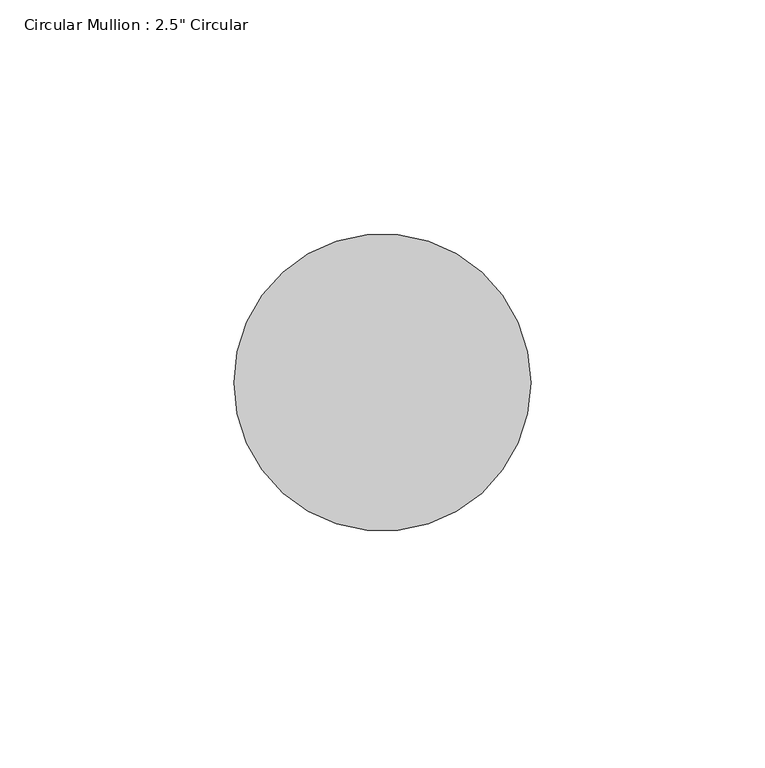
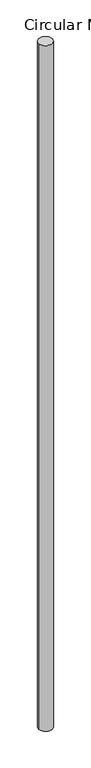
"""IFC4 building model written with IfcOpenShell, lengths in millimetres: member geometry."""

from ifc_helpers import new_model, si_unit, point, frame, frame_2d, origin, place, context, project, spatial, circle_curve, trimmed, segment, composite_curve, outline, extrude, source, transform, mapped, element, save


def member_e759e848(model_context):
    return source(origin(), model_context, "Body", "SweptSolid", [
        extrude(outline(composite_curve([segment(trimmed(circle_curve(frame_2d((-31.75, 0.0)), 31.75), [point((0.0, 0.0))], [point((-63.5, 0.0))], False, "CARTESIAN"), True, "CONTINUOUS"), segment(trimmed(circle_curve(frame_2d((-31.75, 0.0)), 31.75), [point((-63.5, 0.0))], [point((0.0, 0.0))], False, "CARTESIAN"), True, "CONTINUOUS")], self_intersect=False)), frame((0.0, 0.0, -3351.6454545), z_axis=(0.0, 0.0, 1.0), x_axis=(1.0, 0.0, 0.0)), (0.0, 0.0, 1.0), 3351.6454545),
    ])


if __name__ == "__main__":
    model = new_model("IFC4")
    model_context = context("Model", 3, world=origin())
    ifc_project = project(units=[si_unit("LENGTHUNIT", "METRE", prefix="MILLI")], contexts=[model_context])
    site = spatial("IfcSite", under=ifc_project)
    building = spatial("IfcBuilding", under=site)
    placement = place(None, origin())
    member_shape = member_e759e848(model_context)
    element("IfcMember", 1, ObjectType="Circular Mullion : 2.5\" Circular", at=placement, inside=building, context=model_context, shape_type="MappedRepresentation", body=[
        mapped(member_shape, transform((0.0, 0.0, 0.0), x_axis=(1.0, 0.0, 0.0), y_axis=(0.0, 1.0, 0.0), z_axis=(0.0, 0.0, 1.0))),
    ])
    save(model, "model.ifc")

# Revit data of these elements
# Type "Circular Mullion : 2.5\" Circular"
#   built-in parameter 1007350 = 0.104167 (stored number, unit not read)
# Element 1 (IfcMember, "Circular Mullion : 2.5\" Circular")
#   Materials on its faces: "Aluminum"
# Materials
#   "Aluminum": class "Metal", colour RGB 247 247 247, transparency 0, Description = "Aluminum 6061", Cost = 0
